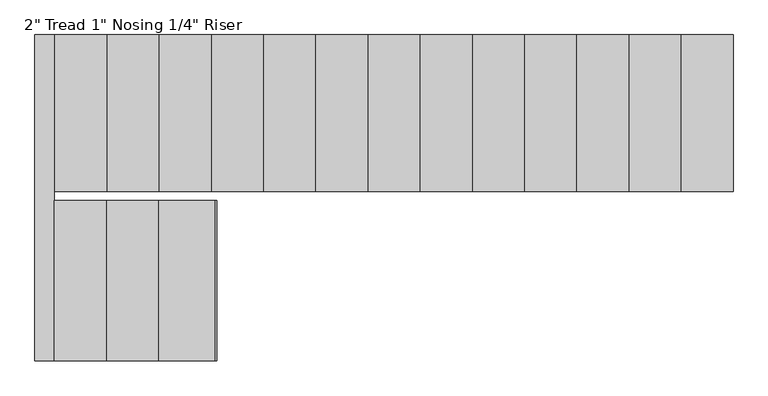
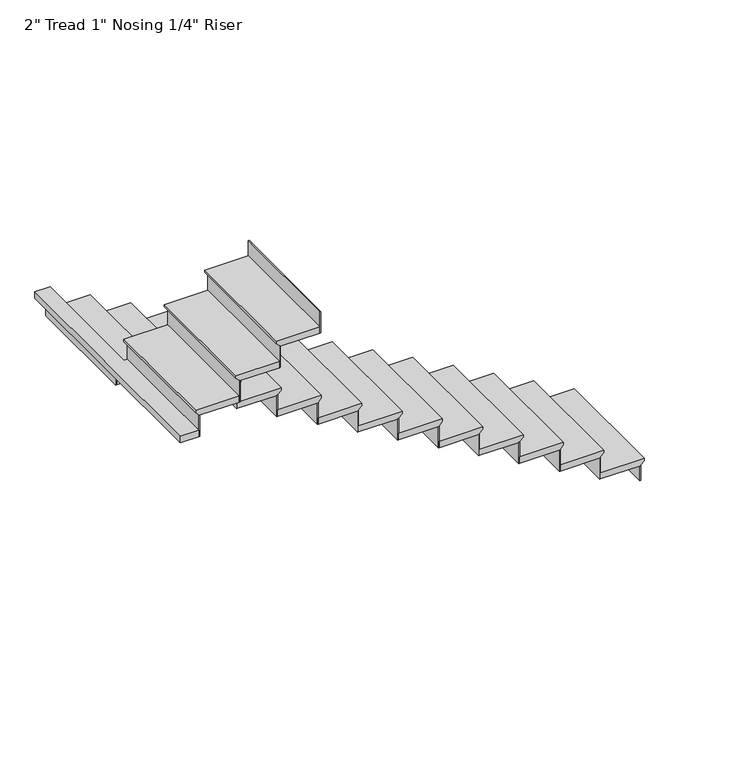
"""IFC4 building model written with IfcOpenShell, lengths in millimetres: stair flight geometry."""

from ifc_helpers import new_model, si_unit, origin, place, context, project, spatial, faceted_brep, source, transform, mapped, element, save


def stair_flight_f65a8a44(model_context):
    return source(origin(), model_context, "Body", "Brep", [
        faceted_brep([(6794.5, 11386.0372886, 12342.2833333), (6794.5, 11386.0372886, 12361.3333333), (6794.5, 10471.6372886, 12361.3333333), (6794.5, 10471.6372886, 12342.2833333), (6769.1, 11386.0372886, 12316.8833333), (6769.1, 10471.6372886, 12316.8833333), (6464.3, 11386.0372886, 12361.3333333), (6464.3, 10471.6372886, 12361.3333333), (6769.1, 10471.6372886, 12310.5333333), (6464.3, 10471.6372886, 12310.5333333), (6464.3, 11386.0372886, 12310.5333333), (6769.1, 11386.0372886, 12310.5333333)], [[[0, 1, 2, 3]], [[4, 0, 3, 5]], [[2, 1, 6, 7]], [[8, 9, 10, 11]], [[2, 7, 9, 8, 5, 3]], [[8, 11, 4, 5]], [[6, 1, 0, 4, 11, 10]], [[7, 6, 10, 9]]]),
        faceted_brep([(6769.1, 11386.0372886, 12310.5333333), (6769.1, 11386.0372886, 12192.0), (6762.75, 11386.0372886, 12192.0), (6762.75, 11386.0372886, 12310.5333333), (6769.1, 10471.6372886, 12310.5333333), (6762.75, 10471.6372886, 12310.5333333), (6762.75, 10471.6372886, 12192.0), (6769.1, 10471.6372886, 12192.0)], [[[0, 1, 2, 3]], [[4, 5, 6, 7]], [[1, 0, 4, 7]], [[2, 1, 7, 6]], [[3, 2, 6, 5]], [[0, 3, 5, 4]]]),
        faceted_brep([(6464.3, 11386.0372886, 12479.8666667), (6464.3, 11386.0372886, 12310.5333333), (6457.95, 11386.0372886, 12310.5333333), (6457.95, 11386.0372886, 12479.8666667), (6464.3, 10471.6372886, 12479.8666667), (6457.95, 10471.6372886, 12479.8666667), (6457.95, 10471.6372886, 12310.5333333), (6464.3, 10471.6372886, 12310.5333333)], [[[0, 1, 2, 3]], [[4, 5, 6, 7]], [[1, 0, 4, 7]], [[2, 1, 7, 6]], [[3, 2, 6, 5]], [[0, 3, 5, 4]]]),
        faceted_brep([(6489.7, 10471.6372886, 12530.6666667), (6489.7, 11386.0372886, 12530.6666667), (6159.5, 11386.0372886, 12530.6666667), (6159.5, 10471.6372886, 12530.6666667), (6464.3, 10471.6372886, 12479.8666667), (6159.5, 10471.6372886, 12479.8666667), (6159.5, 11386.0372886, 12479.8666667), (6464.3, 11386.0372886, 12479.8666667), (6464.3, 10471.6372886, 12486.2166667), (6489.7, 10471.6372886, 12511.6166667), (6464.3, 11386.0372886, 12486.2166667), (6489.7, 11386.0372886, 12511.6166667)], [[[0, 1, 2, 3]], [[4, 5, 6, 7]], [[0, 3, 5, 4, 8, 9]], [[4, 7, 10, 8]], [[2, 1, 11, 10, 7, 6]], [[3, 2, 6, 5]], [[11, 1, 0, 9]], [[10, 11, 9, 8]]]),
        faceted_brep([(6159.5, 11386.0372886, 12649.2), (6159.5, 11386.0372886, 12479.8666667), (6153.15, 11386.0372886, 12479.8666667), (6153.15, 11386.0372886, 12649.2), (6159.5, 10471.6372886, 12649.2), (6153.15, 10471.6372886, 12649.2), (6153.15, 10471.6372886, 12479.8666667), (6159.5, 10471.6372886, 12479.8666667)], [[[0, 1, 2, 3]], [[4, 5, 6, 7]], [[1, 0, 4, 7]], [[2, 1, 7, 6]], [[3, 2, 6, 5]], [[0, 3, 5, 4]]]),
        faceted_brep([(6184.9, 10471.6372886, 12700.0), (6184.9, 11386.0372886, 12700.0), (5854.7, 11386.0372886, 12700.0), (5854.7, 10471.6372886, 12700.0), (6159.5, 10471.6372886, 12649.2), (5854.7, 10471.6372886, 12649.2), (5854.7, 11386.0372886, 12649.2), (6159.5, 11386.0372886, 12649.2), (6159.5, 10471.6372886, 12655.55), (6184.9, 10471.6372886, 12680.95), (6159.5, 11386.0372886, 12655.55), (6184.9, 11386.0372886, 12680.95)], [[[0, 1, 2, 3]], [[4, 5, 6, 7]], [[0, 3, 5, 4, 8, 9]], [[4, 7, 10, 8]], [[2, 1, 11, 10, 7, 6]], [[3, 2, 6, 5]], [[11, 1, 0, 9]], [[10, 11, 9, 8]]]),
        faceted_brep([(5854.7, 11386.0372886, 12818.5333333), (5854.7, 11386.0372886, 12649.2), (5848.35, 11386.0372886, 12649.2), (5848.35, 11386.0372886, 12818.5333333), (5854.7, 10471.6372886, 12818.5333333), (5848.35, 10471.6372886, 12818.5333333), (5848.35, 10471.6372886, 12649.2), (5854.7, 10471.6372886, 12649.2)], [[[0, 1, 2, 3]], [[4, 5, 6, 7]], [[1, 0, 4, 7]], [[2, 1, 7, 6]], [[3, 2, 6, 5]], [[0, 3, 5, 4]]]),
        faceted_brep([(5880.1, 10471.6372886, 12869.3333333), (5880.1, 11386.0372886, 12869.3333333), (5549.9, 11386.0372886, 12869.3333333), (5549.9, 10471.6372886, 12869.3333333), (5854.7, 10471.6372886, 12818.5333333), (5549.9, 10471.6372886, 12818.5333333), (5549.9, 11386.0372886, 12818.5333333), (5854.7, 11386.0372886, 12818.5333333), (5854.7, 10471.6372886, 12824.8833333), (5880.1, 10471.6372886, 12850.2833333), (5854.7, 11386.0372886, 12824.8833333), (5880.1, 11386.0372886, 12850.2833333)], [[[0, 1, 2, 3]], [[4, 5, 6, 7]], [[0, 3, 5, 4, 8, 9]], [[4, 7, 10, 8]], [[2, 1, 11, 10, 7, 6]], [[3, 2, 6, 5]], [[11, 1, 0, 9]], [[10, 11, 9, 8]]]),
        faceted_brep([(5549.9, 11386.0372886, 12987.8666667), (5549.9, 11386.0372886, 12818.5333333), (5543.55, 11386.0372886, 12818.5333333), (5543.55, 11386.0372886, 12987.8666667), (5549.9, 10471.6372886, 12987.8666667), (5543.55, 10471.6372886, 12987.8666667), (5543.55, 10471.6372886, 12818.5333333), (5549.9, 10471.6372886, 12818.5333333)], [[[0, 1, 2, 3]], [[4, 5, 6, 7]], [[1, 0, 4, 7]], [[2, 1, 7, 6]], [[3, 2, 6, 5]], [[0, 3, 5, 4]]]),
        faceted_brep([(5575.3, 10471.6372886, 13038.6666667), (5575.3, 11386.0372886, 13038.6666667), (5245.1, 11386.0372886, 13038.6666667), (5245.1, 10471.6372886, 13038.6666667), (5549.9, 10471.6372886, 12987.8666667), (5245.1, 10471.6372886, 12987.8666667), (5245.1, 11386.0372886, 12987.8666667), (5549.9, 11386.0372886, 12987.8666667), (5549.9, 10471.6372886, 12994.2166667), (5575.3, 10471.6372886, 13019.6166667), (5549.9, 11386.0372886, 12994.2166667), (5575.3, 11386.0372886, 13019.6166667)], [[[0, 1, 2, 3]], [[4, 5, 6, 7]], [[0, 3, 5, 4, 8, 9]], [[4, 7, 10, 8]], [[2, 1, 11, 10, 7, 6]], [[3, 2, 6, 5]], [[11, 1, 0, 9]], [[10, 11, 9, 8]]]),
        faceted_brep([(5245.1, 11386.0372886, 13157.2), (5245.1, 11386.0372886, 12987.8666667), (5238.75, 11386.0372886, 12987.8666667), (5238.75, 11386.0372886, 13157.2), (5245.1, 10471.6372886, 13157.2), (5238.75, 10471.6372886, 13157.2), (5238.75, 10471.6372886, 12987.8666667), (5245.1, 10471.6372886, 12987.8666667)], [[[0, 1, 2, 3]], [[4, 5, 6, 7]], [[1, 0, 4, 7]], [[2, 1, 7, 6]], [[3, 2, 6, 5]], [[0, 3, 5, 4]]]),
        faceted_brep([(5270.5, 10471.6372886, 13208.0), (5270.5, 11386.0372886, 13208.0), (4940.3, 11386.0372886, 13208.0), (4940.3, 10471.6372886, 13208.0), (5245.1, 10471.6372886, 13157.2), (4940.3, 10471.6372886, 13157.2), (4940.3, 11386.0372886, 13157.2), (5245.1, 11386.0372886, 13157.2), (5245.1, 10471.6372886, 13163.55), (5270.5, 10471.6372886, 13188.95), (5245.1, 11386.0372886, 13163.55), (5270.5, 11386.0372886, 13188.95)], [[[0, 1, 2, 3]], [[4, 5, 6, 7]], [[0, 3, 5, 4, 8, 9]], [[4, 7, 10, 8]], [[2, 1, 11, 10, 7, 6]], [[3, 2, 6, 5]], [[11, 1, 0, 9]], [[10, 11, 9, 8]]]),
        faceted_brep([(4940.3, 11386.0372886, 13326.5333333), (4940.3, 11386.0372886, 13157.2), (4933.95, 11386.0372886, 13157.2), (4933.95, 11386.0372886, 13326.5333333), (4940.3, 10471.6372886, 13326.5333333), (4933.95, 10471.6372886, 13326.5333333), (4933.95, 10471.6372886, 13157.2), (4940.3, 10471.6372886, 13157.2)], [[[0, 1, 2, 3]], [[4, 5, 6, 7]], [[1, 0, 4, 7]], [[2, 1, 7, 6]], [[3, 2, 6, 5]], [[0, 3, 5, 4]]]),
        faceted_brep([(4965.7, 10471.6372886, 13377.3333333), (4965.7, 11386.0372886, 13377.3333333), (4635.5, 11386.0372886, 13377.3333333), (4635.5, 10471.6372886, 13377.3333333), (4940.3, 10471.6372886, 13326.5333333), (4635.5, 10471.6372886, 13326.5333333), (4635.5, 11386.0372886, 13326.5333333), (4940.3, 11386.0372886, 13326.5333333), (4940.3, 10471.6372886, 13332.8833333), (4965.7, 10471.6372886, 13358.2833333), (4940.3, 11386.0372886, 13332.8833333), (4965.7, 11386.0372886, 13358.2833333)], [[[0, 1, 2, 3]], [[4, 5, 6, 7]], [[0, 3, 5, 4, 8, 9]], [[4, 7, 10, 8]], [[2, 1, 11, 10, 7, 6]], [[3, 2, 6, 5]], [[11, 1, 0, 9]], [[10, 11, 9, 8]]]),
        faceted_brep([(4635.5, 11386.0372886, 13495.8666667), (4635.5, 11386.0372886, 13326.5333333), (4629.15, 11386.0372886, 13326.5333333), (4629.15, 11386.0372886, 13495.8666667), (4635.5, 10471.6372886, 13495.8666667), (4629.15, 10471.6372886, 13495.8666667), (4629.15, 10471.6372886, 13326.5333333), (4635.5, 10471.6372886, 13326.5333333)], [[[0, 1, 2, 3]], [[4, 5, 6, 7]], [[1, 0, 4, 7]], [[2, 1, 7, 6]], [[3, 2, 6, 5]], [[0, 3, 5, 4]]]),
        faceted_brep([(4660.9, 10471.6372886, 13546.6666667), (4660.9, 11386.0372886, 13546.6666667), (4330.7, 11386.0372886, 13546.6666667), (4330.7, 10471.6372886, 13546.6666667), (4635.5, 10471.6372886, 13495.8666667), (4330.7, 10471.6372886, 13495.8666667), (4330.7, 11386.0372886, 13495.8666667), (4635.5, 11386.0372886, 13495.8666667), (4635.5, 10471.6372886, 13502.2166667), (4660.9, 10471.6372886, 13527.6166667), (4635.5, 11386.0372886, 13502.2166667), (4660.9, 11386.0372886, 13527.6166667)], [[[0, 1, 2, 3]], [[4, 5, 6, 7]], [[0, 3, 5, 4, 8, 9]], [[4, 7, 10, 8]], [[2, 1, 11, 10, 7, 6]], [[3, 2, 6, 5]], [[11, 1, 0, 9]], [[10, 11, 9, 8]]]),
        faceted_brep([(4330.7, 11386.0372886, 13665.2), (4330.7, 11386.0372886, 13495.8666667), (4324.35, 11386.0372886, 13495.8666667), (4324.35, 11386.0372886, 13665.2), (4330.7, 10471.6372886, 13665.2), (4324.35, 10471.6372886, 13665.2), (4324.35, 10471.6372886, 13495.8666667), (4330.7, 10471.6372886, 13495.8666667)], [[[0, 1, 2, 3]], [[4, 5, 6, 7]], [[1, 0, 4, 7]], [[2, 1, 7, 6]], [[3, 2, 6, 5]], [[0, 3, 5, 4]]]),
        faceted_brep([(4356.1, 10471.6372886, 13716.0), (4356.1, 11386.0372886, 13716.0), (4025.9, 11386.0372886, 13716.0), (4025.9, 10471.6372886, 13716.0), (4330.7, 10471.6372886, 13665.2), (4025.9, 10471.6372886, 13665.2), (4025.9, 11386.0372886, 13665.2), (4330.7, 11386.0372886, 13665.2), (4330.7, 10471.6372886, 13671.55), (4356.1, 10471.6372886, 13696.95), (4330.7, 11386.0372886, 13671.55), (4356.1, 11386.0372886, 13696.95)], [[[0, 1, 2, 3]], [[4, 5, 6, 7]], [[0, 3, 5, 4, 8, 9]], [[4, 7, 10, 8]], [[2, 1, 11, 10, 7, 6]], [[3, 2, 6, 5]], [[11, 1, 0, 9]], [[10, 11, 9, 8]]]),
        faceted_brep([(4025.9, 11386.0372886, 13834.5333333), (4025.9, 11386.0372886, 13665.2), (4019.55, 11386.0372886, 13665.2), (4019.55, 11386.0372886, 13834.5333333), (4025.9, 10471.6372886, 13834.5333333), (4019.55, 10471.6372886, 13834.5333333), (4019.55, 10471.6372886, 13665.2), (4025.9, 10471.6372886, 13665.2)], [[[0, 1, 2, 3]], [[4, 5, 6, 7]], [[1, 0, 4, 7]], [[2, 1, 7, 6]], [[3, 2, 6, 5]], [[0, 3, 5, 4]]]),
        faceted_brep([(4051.3, 10471.6372886, 13885.3333333), (4051.3, 11386.0372886, 13885.3333333), (3721.1, 11386.0372886, 13885.3333333), (3721.1, 10471.6372886, 13885.3333333), (4025.9, 10471.6372886, 13834.5333333), (3721.1, 10471.6372886, 13834.5333333), (3721.1, 11386.0372886, 13834.5333333), (4025.9, 11386.0372886, 13834.5333333), (4025.9, 10471.6372886, 13840.8833333), (4051.3, 10471.6372886, 13866.2833333), (4025.9, 11386.0372886, 13840.8833333), (4051.3, 11386.0372886, 13866.2833333)], [[[0, 1, 2, 3]], [[4, 5, 6, 7]], [[0, 3, 5, 4, 8, 9]], [[4, 7, 10, 8]], [[2, 1, 11, 10, 7, 6]], [[3, 2, 6, 5]], [[11, 1, 0, 9]], [[10, 11, 9, 8]]]),
        faceted_brep([(3721.1, 11386.0372886, 14003.8666667), (3721.1, 11386.0372886, 13834.5333333), (3714.75, 11386.0372886, 13834.5333333), (3714.75, 11386.0372886, 14003.8666667), (3721.1, 10471.6372886, 14003.8666667), (3714.75, 10471.6372886, 14003.8666667), (3714.75, 10471.6372886, 13834.5333333), (3721.1, 10471.6372886, 13834.5333333)], [[[0, 1, 2, 3]], [[4, 5, 6, 7]], [[1, 0, 4, 7]], [[2, 1, 7, 6]], [[3, 2, 6, 5]], [[0, 3, 5, 4]]]),
        faceted_brep([(3746.5, 10471.6372886, 14054.6666667), (3746.5, 11386.0372886, 14054.6666667), (3416.3, 11386.0372886, 14054.6666667), (3416.3, 10471.6372886, 14054.6666667), (3721.1, 10471.6372886, 14003.8666667), (3416.3, 10471.6372886, 14003.8666667), (3416.3, 11386.0372886, 14003.8666667), (3721.1, 11386.0372886, 14003.8666667), (3721.1, 10471.6372886, 14010.2166667), (3746.5, 10471.6372886, 14035.6166667), (3721.1, 11386.0372886, 14010.2166667), (3746.5, 11386.0372886, 14035.6166667)], [[[0, 1, 2, 3]], [[4, 5, 6, 7]], [[0, 3, 5, 4, 8, 9]], [[4, 7, 10, 8]], [[2, 1, 11, 10, 7, 6]], [[3, 2, 6, 5]], [[11, 1, 0, 9]], [[10, 11, 9, 8]]]),
        faceted_brep([(3416.3, 11386.0372886, 14173.2), (3416.3, 11386.0372886, 14003.8666667), (3409.95, 11386.0372886, 14003.8666667), (3409.95, 11386.0372886, 14173.2), (3416.3, 10471.6372886, 14173.2), (3409.95, 10471.6372886, 14173.2), (3409.95, 10471.6372886, 14003.8666667), (3416.3, 10471.6372886, 14003.8666667)], [[[0, 1, 2, 3]], [[4, 5, 6, 7]], [[1, 0, 4, 7]], [[2, 1, 7, 6]], [[3, 2, 6, 5]], [[0, 3, 5, 4]]]),
        faceted_brep([(3441.7, 10471.6372886, 14224.0), (3441.7, 11386.0372886, 14224.0), (3111.5, 11386.0372886, 14224.0), (3111.5, 10471.6372886, 14224.0), (3416.3, 10471.6372886, 14173.2), (3111.5, 10471.6372886, 14173.2), (3111.5, 11386.0372886, 14173.2), (3416.3, 11386.0372886, 14173.2), (3416.3, 10471.6372886, 14179.55), (3441.7, 10471.6372886, 14204.95), (3416.3, 11386.0372886, 14179.55), (3441.7, 11386.0372886, 14204.95)], [[[0, 1, 2, 3]], [[4, 5, 6, 7]], [[0, 3, 5, 4, 8, 9]], [[4, 7, 10, 8]], [[2, 1, 11, 10, 7, 6]], [[3, 2, 6, 5]], [[11, 1, 0, 9]], [[10, 11, 9, 8]]]),
        faceted_brep([(3111.5, 11386.0372886, 14342.5333333), (3111.5, 11386.0372886, 14173.2), (3105.15, 11386.0372886, 14173.2), (3105.15, 11386.0372886, 14342.5333333), (3111.5, 10471.6372886, 14342.5333333), (3105.15, 10471.6372886, 14342.5333333), (3105.15, 10471.6372886, 14173.2), (3111.5, 10471.6372886, 14173.2)], [[[0, 1, 2, 3]], [[4, 5, 6, 7]], [[1, 0, 4, 7]], [[2, 1, 7, 6]], [[3, 2, 6, 5]], [[0, 3, 5, 4]]]),
        faceted_brep([(3136.9, 10471.6372886, 14393.3333333), (3136.9, 11386.0372886, 14393.3333333), (2806.7, 11386.0372886, 14393.3333333), (2806.7, 10471.6372886, 14393.3333333), (3111.5, 10471.6372886, 14342.5333333), (2806.7, 10471.6372886, 14342.5333333), (2806.7, 11386.0372886, 14342.5333333), (3111.5, 11386.0372886, 14342.5333333), (3111.5, 10471.6372886, 14348.8833333), (3136.9, 10471.6372886, 14374.2833333), (3111.5, 11386.0372886, 14348.8833333), (3136.9, 11386.0372886, 14374.2833333)], [[[0, 1, 2, 3]], [[4, 5, 6, 7]], [[0, 3, 5, 4, 8, 9]], [[4, 7, 10, 8]], [[2, 1, 11, 10, 7, 6]], [[3, 2, 6, 5]], [[11, 1, 0, 9]], [[10, 11, 9, 8]]]),
        faceted_brep([(2806.7, 11386.0372886, 14511.8666667), (2806.7, 11386.0372886, 14342.5333333), (2800.35, 11386.0372886, 14342.5333333), (2800.35, 11386.0372886, 14511.8666667), (2806.7, 10471.6372886, 14511.8666667), (2800.35, 10471.6372886, 14511.8666667), (2800.35, 10471.6372886, 14342.5333333), (2806.7, 10471.6372886, 14342.5333333)], [[[0, 1, 2, 3]], [[4, 5, 6, 7]], [[1, 0, 4, 7]], [[2, 1, 7, 6]], [[3, 2, 6, 5]], [[0, 3, 5, 4]]]),
        faceted_brep([(2857.5, 10418.2972886, 14562.6666667), (2832.1, 10418.2972886, 14562.6666667), (2832.1, 11386.0372886, 14562.6666667), (2717.8, 11386.0372886, 14562.6666667), (2717.8, 9481.0372886, 14562.6666667), (2857.5, 9481.0372886, 14562.6666667), (2832.1, 10418.2972886, 14511.8666667), (2857.5, 10418.2972886, 14511.8666667), (2857.5, 9481.0372886, 14511.8666667), (2717.8, 9481.0372886, 14511.8666667), (2717.8, 11386.0372886, 14511.8666667), (2806.7, 11386.0372886, 14511.8666667), (2806.7, 10471.6372886, 14511.8666667), (2832.1, 10471.6372886, 14511.8666667), (2832.1, 10471.6372886, 14543.6166667), (2832.1, 11386.0372886, 14543.6166667), (2806.7, 10471.6372886, 14518.2166667), (2806.7, 11386.0372886, 14518.2166667)], [[[0, 1, 2, 3, 4, 5]], [[6, 7, 8, 9, 10, 11, 12, 13]], [[1, 0, 7, 6]], [[2, 1, 6, 13, 14, 15]], [[13, 12, 16, 14]], [[12, 11, 17, 16]], [[3, 2, 15, 17, 11, 10]], [[4, 3, 10, 9]], [[5, 4, 9, 8]], [[0, 5, 8, 7]], [[17, 15, 14, 16]]]),
        faceted_brep([(2857.5, 9481.0372886, 14681.2), (2857.5, 9481.0372886, 14511.8666667), (2863.85, 9481.0372886, 14511.8666667), (2863.85, 9481.0372886, 14681.2), (2857.5, 10418.2972886, 14681.2), (2863.85, 10418.2972886, 14681.2), (2863.85, 10418.2972886, 14511.8666667), (2857.5, 10418.2972886, 14511.8666667)], [[[0, 1, 2, 3]], [[4, 5, 6, 7]], [[1, 0, 4, 7]], [[2, 1, 7, 6]], [[3, 2, 6, 5]], [[0, 3, 5, 4]]]),
        faceted_brep([(2832.1, 10418.2972886, 14732.0), (2832.1, 9481.0372886, 14732.0), (3162.3, 9481.0372886, 14732.0), (3162.3, 10418.2972886, 14732.0), (2857.5, 10418.2972886, 14681.2), (3162.3, 10418.2972886, 14681.2), (3162.3, 9481.0372886, 14681.2), (2857.5, 9481.0372886, 14681.2), (2857.5, 10418.2972886, 14687.55), (2832.1, 10418.2972886, 14712.95), (2857.5, 9481.0372886, 14687.55), (2832.1, 9481.0372886, 14712.95)], [[[0, 1, 2, 3]], [[4, 5, 6, 7]], [[0, 3, 5, 4, 8, 9]], [[4, 7, 10, 8]], [[2, 1, 11, 10, 7, 6]], [[3, 2, 6, 5]], [[11, 1, 0, 9]], [[10, 11, 9, 8]]]),
        faceted_brep([(3162.3, 9481.0372886, 14850.5333333), (3162.3, 9481.0372886, 14681.2), (3168.65, 9481.0372886, 14681.2), (3168.65, 9481.0372886, 14850.5333333), (3162.3, 10418.2972886, 14850.5333333), (3168.65, 10418.2972886, 14850.5333333), (3168.65, 10418.2972886, 14681.2), (3162.3, 10418.2972886, 14681.2)], [[[0, 1, 2, 3]], [[4, 5, 6, 7]], [[1, 0, 4, 7]], [[2, 1, 7, 6]], [[3, 2, 6, 5]], [[0, 3, 5, 4]]]),
        faceted_brep([(3136.9, 10418.2972886, 14901.3333333), (3136.9, 9481.0372886, 14901.3333333), (3467.1, 9481.0372886, 14901.3333333), (3467.1, 10418.2972886, 14901.3333333), (3162.3, 10418.2972886, 14850.5333333), (3467.1, 10418.2972886, 14850.5333333), (3467.1, 9481.0372886, 14850.5333333), (3162.3, 9481.0372886, 14850.5333333), (3162.3, 10418.2972886, 14856.8833333), (3136.9, 10418.2972886, 14882.2833333), (3162.3, 9481.0372886, 14856.8833333), (3136.9, 9481.0372886, 14882.2833333)], [[[0, 1, 2, 3]], [[4, 5, 6, 7]], [[0, 3, 5, 4, 8, 9]], [[4, 7, 10, 8]], [[2, 1, 11, 10, 7, 6]], [[3, 2, 6, 5]], [[11, 1, 0, 9]], [[10, 11, 9, 8]]]),
        faceted_brep([(3467.1, 9481.0372886, 15019.8666667), (3467.1, 9481.0372886, 14850.5333333), (3473.45, 9481.0372886, 14850.5333333), (3473.45, 9481.0372886, 15019.8666667), (3467.1, 10418.2972886, 15019.8666667), (3473.45, 10418.2972886, 15019.8666667), (3473.45, 10418.2972886, 14850.5333333), (3467.1, 10418.2972886, 14850.5333333)], [[[0, 1, 2, 3]], [[4, 5, 6, 7]], [[1, 0, 4, 7]], [[2, 1, 7, 6]], [[3, 2, 6, 5]], [[0, 3, 5, 4]]]),
        faceted_brep([(3771.9019847, 9481.0372886, 15189.2), (3771.9019847, 9481.0372886, 15019.8666667), (3778.2519847, 9481.0372886, 15019.8666667), (3778.2519847, 9481.0372886, 15189.2), (3771.9019847, 10418.2972886, 15189.2), (3778.2519847, 10418.2972886, 15189.2), (3778.2519847, 10418.2972886, 15019.8666667), (3771.9019847, 10418.2972886, 15019.8666667)], [[[0, 1, 2, 3]], [[4, 5, 6, 7]], [[1, 0, 4, 7]], [[2, 1, 7, 6]], [[3, 2, 6, 5]], [[0, 3, 5, 4]]]),
        faceted_brep([(3441.7, 10418.2972886, 15070.6666667), (3441.7, 9481.0372886, 15070.6666667), (3771.9019847, 9481.0372886, 15070.6666667), (3771.9019847, 10418.2972886, 15070.6666667), (3467.1, 10418.2972886, 15019.8666667), (3771.9019847, 10418.2972886, 15019.8666667), (3771.9019847, 9481.0372886, 15019.8666667), (3467.1, 9481.0372886, 15019.8666667), (3467.1, 10418.2972886, 15026.2166667), (3441.7, 10418.2972886, 15051.6166667), (3467.1, 9481.0372886, 15026.2166667), (3441.7, 9481.0372886, 15051.6166667)], [[[0, 1, 2, 3]], [[4, 5, 6, 7]], [[0, 3, 5, 4, 8, 9]], [[4, 7, 10, 8]], [[2, 1, 11, 10, 7, 6]], [[3, 2, 6, 5]], [[11, 1, 0, 9]], [[10, 11, 9, 8]]]),
    ])


if __name__ == "__main__":
    model = new_model("IFC4")
    model_context = context("Model", 3, world=origin())
    ifc_project = project(units=[si_unit("LENGTHUNIT", "METRE", prefix="MILLI")], contexts=[model_context])
    site = spatial("IfcSite", under=ifc_project)
    building = spatial("IfcBuilding", under=site)
    placement = place(None, origin())
    stair_flight_shape = stair_flight_f65a8a44(model_context)
    element("IfcStairFlight", 1, ObjectType="2\" Tread 1\" Nosing 1/4\" Riser", at=placement, inside=building, context=model_context, shape_type="MappedRepresentation", body=[
        mapped(stair_flight_shape, transform((0.0, 0.0, 0.0), x_axis=(1.0, 0.0, 0.0), y_axis=(0.0, 1.0, 0.0), z_axis=(0.0, 0.0, 1.0))),
    ])
    save(model, "model.ifc")
